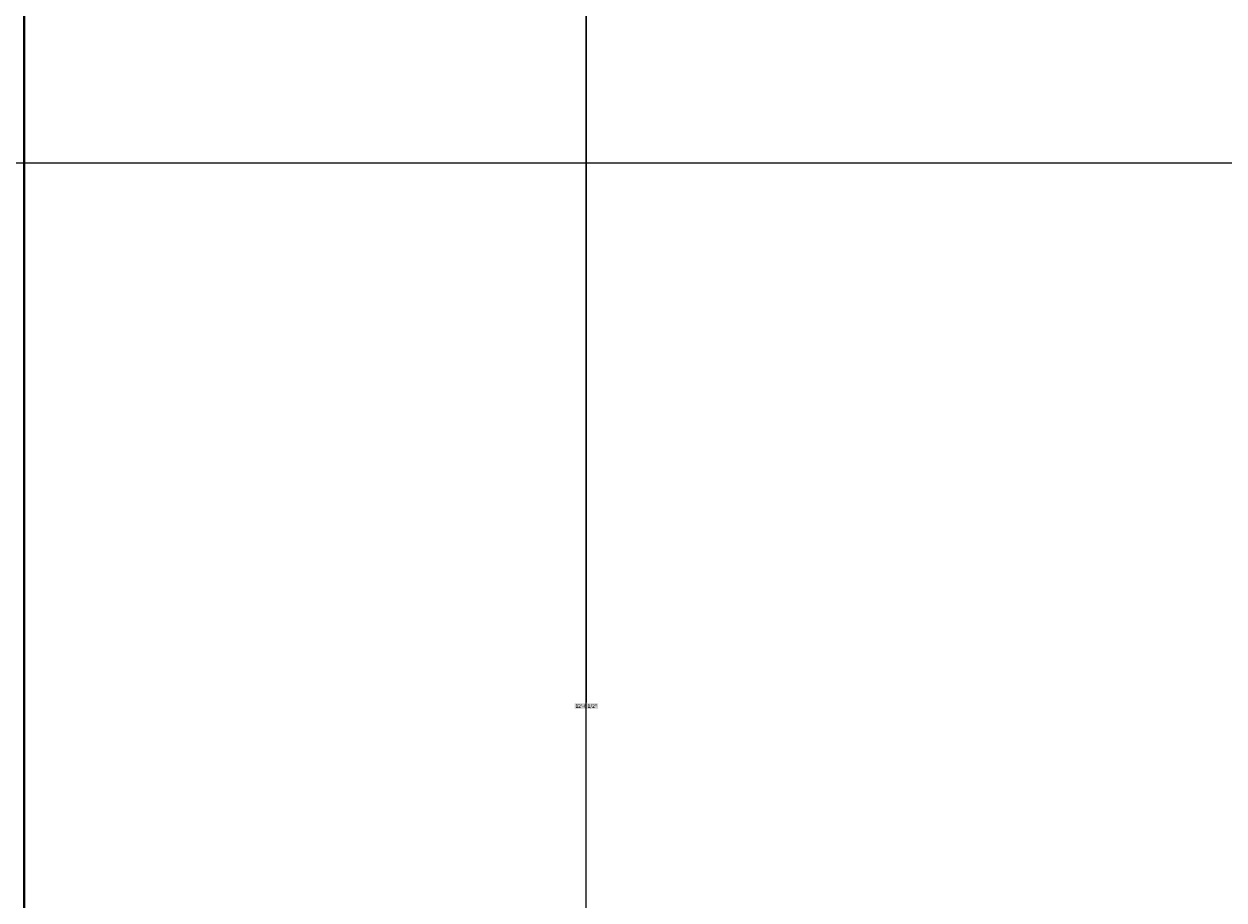
# Model space of a CAD drawing. Units: inches. Extents: x -301 to 715, y -607 to 364.
# Tile 94 of 141: x 133 to 194, y -168 to -124. Entities that reach past the tile are written whole.
import ezdxf

# ---------------------------------------------------------------- set-up
doc = ezdxf.new("R2010")
doc.units = ezdxf.units.IN
doc.header["$MEASUREMENT"] = 0
doc.layers.add('A-ANNO-DIMS', color=2, linetype='Continuous', lineweight=18)
doc.layers.add('A-WALL', color=3, linetype='Continuous', lineweight=40)
doc.styles.get("Standard").update_dxf_attribs({"font": 'arial.ttf'})
doc.dimstyles.get("Standard").update_dxf_attribs({"dimtxt": 0.18, "dimasz": 0.18, "dimexe": 0.18, "dimexo": 0.0625, "dimgap": 0.09, "dimtad": 0, "dimtih": 1, "dimtoh": 1, "dimdec": 1, "dimzin": 0, "dimdsep": 46, "dimlunit": 4, "dimtxsty": 'Standard', "dimcen": 0.09, "dimclrd": 3, "dimclre": 4, "dimclrt": 6, "dimadec": 0, "dimazin": 0, "dimtfac": 1, "dimtdec": 1, "dimtofl": 0, "dimtmove": 0, "dimatfit": 3, "dimfxl": 1, "dimtfill": 2, "dimtfillclr": 51, "dimtolj": 1, "dimtzin": 0, "dimarcsym": 0})

# ---------------------------------------------------------------- blocks, each defined once
blk = doc.blocks.new('*D152')
at = {"layer": 'A-ANNO-DIMS', "color": 4, "lineweight": -2, "transparency": 16777216}
for p, q in [((123.959, -130.818), (233.659, -130.818)), ((132.959, -223.818), (233.659, -223.818))]:
    blk.add_line(p, q, dxfattribs=at)
at = {"layer": 'A-ANNO-DIMS', "color": 3, "lineweight": -2, "transparency": 16777216}
for p, q in [((233.479, -130.998), (233.479, -177.136)), ((233.479, -223.638), (233.479, -177.5))]:
    blk.add_line(p, q, dxfattribs=at)
at = {"layer": 'A-ANNO-DIMS', "color": 3, "transparency": 16777216}
for points in [[(233.449, -130.998), (233.509, -130.998), (233.479, -130.818)], [(233.449, -223.638), (233.509, -223.638), (233.479, -223.818)]]:
    blk.add_solid(points, dxfattribs=at)
at = {"layer": 'Defpoints', "color": 0, "transparency": 16777216}
for p in [(123.897, -130.818), (233.479, -130.818), (132.897, -223.818)]:
    blk.add_point(p, dxfattribs=at)
at = {"layer": 'A-ANNO-DIMS', "color": 6, "transparency": 16777216, "insert": (233.479, -177.318), "char_height": 0.18, "attachment_point": 5, "bg_fill": 1, "box_fill_scale": 1.25, "bg_fill_color": 51, "bg_fill_transparency": 0}
blk.add_mtext('\\A1;7\'-9"', dxfattribs=at)
blk = doc.blocks.new('*D162')
at = {"layer": 'A-ANNO-DIMS', "color": 4, "lineweight": -2, "transparency": 16777216}
for p, q in [((222.328, 320.182), (161.439, 320.182)), ((222.328, -233.818), (161.439, -233.818))]:
    blk.add_line(p, q, dxfattribs=at)
at = {"layer": 'A-ANNO-DIMS', "color": 3, "lineweight": -2, "transparency": 16777216}
for p, q in [((161.619, 320.002), (161.619, 43.364)), ((161.619, -233.638), (161.619, 43))]:
    blk.add_line(p, q, dxfattribs=at)
at = {"layer": 'A-ANNO-DIMS', "color": 3, "transparency": 16777216}
for points in [[(161.589, 320.002), (161.649, 320.002), (161.619, 320.182)], [(161.589, -233.638), (161.649, -233.638), (161.619, -233.818)]]:
    blk.add_solid(points, dxfattribs=at)
at = {"layer": 'Defpoints', "color": 0, "transparency": 16777216}
for p in [(161.619, 320.182), (222.39, 320.182), (222.39, -233.818)]:
    blk.add_point(p, dxfattribs=at)
at = {"layer": 'A-ANNO-DIMS', "color": 6, "transparency": 16777216, "insert": (161.619, 43.182), "char_height": 0.18, "attachment_point": 5, "bg_fill": 1, "box_fill_scale": 1.25, "bg_fill_color": 51, "bg_fill_transparency": 0}
blk.add_mtext('\\A1;46\'-2"', dxfattribs=at)
blk = doc.blocks.new('*D167')
at = {"layer": 'A-ANNO-DIMS', "color": 4, "lineweight": -2, "transparency": 16777216}
for p, q in [((222.328, -83.318), (161.439, -83.318)), ((222.328, -233.818), (161.439, -233.818))]:
    blk.add_line(p, q, dxfattribs=at)
at = {"layer": 'A-ANNO-DIMS', "color": 3, "lineweight": -2, "transparency": 16777216}
for p, q in [((161.619, -83.498), (161.619, -158.385)), ((161.619, -233.638), (161.619, -158.751))]:
    blk.add_line(p, q, dxfattribs=at)
at = {"layer": 'A-ANNO-DIMS', "color": 3, "transparency": 16777216}
for points in [[(161.589, -83.498), (161.649, -83.498), (161.619, -83.318)], [(161.589, -233.638), (161.649, -233.638), (161.619, -233.818)]]:
    blk.add_solid(points, dxfattribs=at)
at = {"layer": 'Defpoints', "color": 0, "transparency": 16777216}
for p in [(161.619, -83.318), (222.39, -83.318), (222.39, -233.818)]:
    blk.add_point(p, dxfattribs=at)
at = {"layer": 'A-ANNO-DIMS', "color": 6, "transparency": 16777216, "insert": (161.619, -158.568), "char_height": 0.18, "attachment_point": 5, "bg_fill": 1, "box_fill_scale": 1.25, "bg_fill_color": 51, "bg_fill_transparency": 0}
blk.add_mtext('\\A1;12\'-6 1/2"', dxfattribs=at)

msp = doc.modelspace()

# ---------------------------------------------------------------- linework, layer by layer
at = {"layer": 'A-WALL'}
for p, q in [((132.897, -124.818), (132.897, -76.818)), ((132.897, -223.818), (132.897, -124.818))]:
    msp.add_line(p, q, dxfattribs=at)

# ---------------------------------------------------------------- dimensions: what is measured, and where the dimension line sits
at = {"layer": 'A-ANNO-DIMS'}
for base, p1, p2, picture, middle in [((161.619, 320.182), (222.39, -233.818), (222.39, 320.182), '*D162', (161.619, 43.182)), ((161.619, -83.318), (222.39, -233.818), (222.39, -83.318), '*D167', (161.619, -158.568)), ((233.479, -130.818), (132.897, -223.818), (123.897, -130.818), '*D152', (233.479, -177.318))]:
    dim = msp.add_linear_dim(base=base, p1=p1, p2=p2, angle=90, dimstyle='Standard', override={"dimdec": 1, "dimlfac": 1, "dimrnd": 0, "dimzin": 1, "dimdsep": 46, "dimlunit": 4, "dimfrac": 2}, dxfattribs=at)
    dim.commit()
    dim.dimension.update_dxf_attribs({"geometry": picture, "text_midpoint": middle})

doc.saveas('drawing.dxf')
